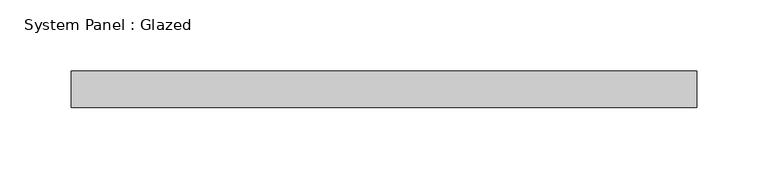
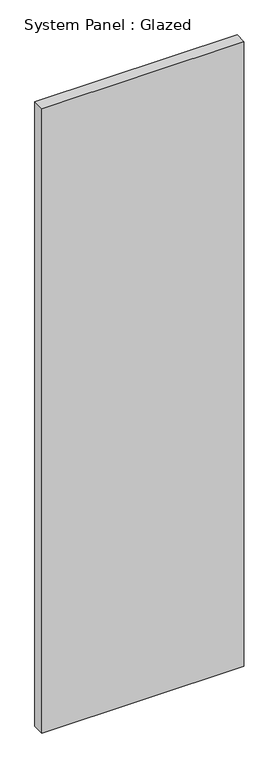
"""IFC4 building model written with IfcOpenShell, lengths in millimetres: plate geometry, System Panel : Glazed."""

from ifc_helpers import new_model, si_unit, origin, origin_with_axes, place, context, project, spatial, polyline, outline, extrude, source, transform, mapped, element, save


def system_panel_glazed_a38fa740(model_context):
    return source(origin(), model_context, "Body", "SweptSolid", [
        extrude(outline(polyline([(219.075, 19.05), (-219.075, 19.05), (-219.075, 44.45), (219.075, 44.45), (219.075, 19.05)])), origin_with_axes(), (0.0, 0.0, 1.0), 1430.3709712),
    ])


if __name__ == "__main__":
    model = new_model("IFC4")
    model_context = context("Model", 3, world=origin())
    ifc_project = project(units=[si_unit("LENGTHUNIT", "METRE", prefix="MILLI")], contexts=[model_context])
    site = spatial("IfcSite", under=ifc_project)
    building = spatial("IfcBuilding", under=site)
    placement = place(None, origin())
    system_panel_glazed_shape = system_panel_glazed_a38fa740(model_context)
    element("IfcPlate", 1, ObjectType="System Panel : Glazed", at=placement, inside=building, context=model_context, shape_type="MappedRepresentation", body=[
        mapped(system_panel_glazed_shape, transform((0.0, 0.0, 0.0), x_axis=(1.0, 0.0, 0.0), y_axis=(0.0, 1.0, 0.0), z_axis=(0.0, 0.0, 1.0))),
    ])
    save(model, "model.ifc")

# Revit data of these elements
# Type "System Panel : Glazed"
#   Construction Type Id = "GSP4R"
#   Analytic Construction = "1/8 in Pilkington single glazing"
#   Visual Light Transmittance = 0.9
#   Solar Heat Gain Coefficient = 0.86
#   Heat Transfer Coefficient (U) = 1.18115 BTU/(h·ft²·°F)
#   Define Thermal Properties by = 1
# Element 1 (IfcPlate, "System Panel : Glazed")
#   Materials on its faces: "Glass"
# Materials
#   "Glass": class "Glass", colour RGB 0 128 192, transparency 0.75, Description = "Soda Lime Glass", Cost = 0
